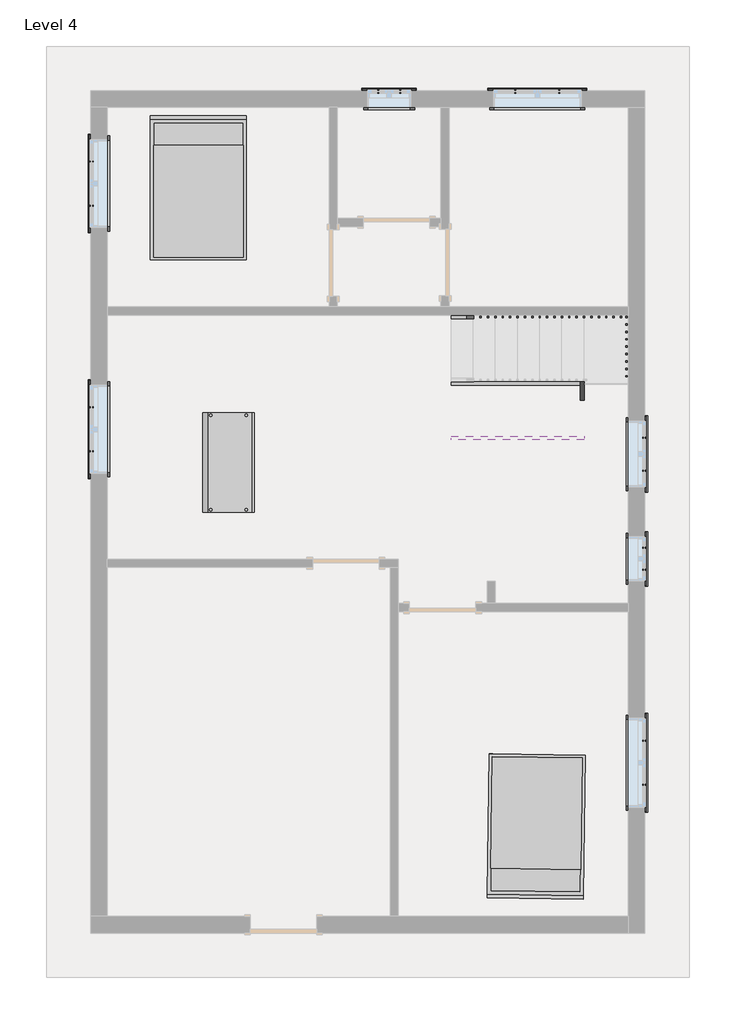
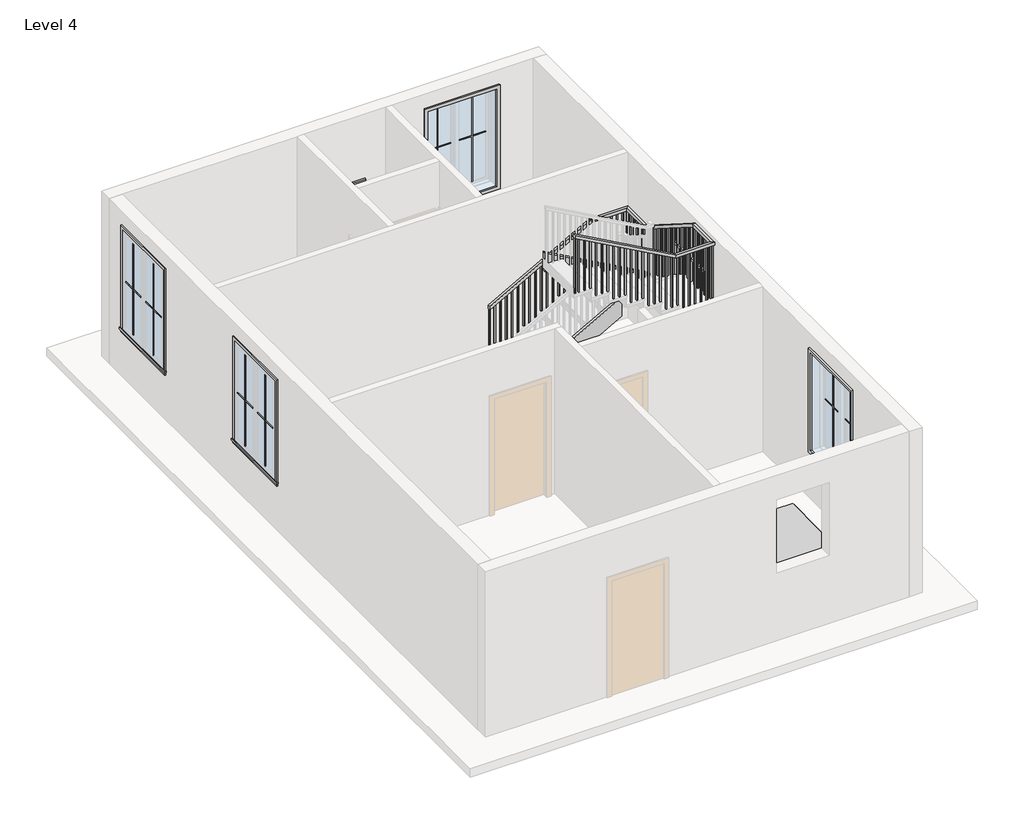
# One storey, part 2 of 2: 29 proxies, 3 members, 2 furniture elements, 1 railing.
"""IFC4 building model written with IfcOpenShell, lengths in millimetres."""

from ifc_helpers import new_model, si_unit, frame, origin, place, context, project, spatial, polyline, outline, extrude, faceted_brep, transform, mapped, element, save
from components import modern_coffee_table_17989_modern_coffee_table_17989_d3a860c8, muntin_pattern_2x2_muntin_pattern_2x2_2b4d9f72, muntin_pattern_2x2_muntin_pattern_2x2_ef995ed3, muntin_pattern_2x2_muntin_pattern_2x2_53152e2c, muntin_pattern_2x2_muntin_pattern_2x2_e8f3e573, muntin_pattern_2x2_muntin_pattern_2x2_9b64c8d5, muntin_pattern_2x2_muntin_pattern_2x2_d319fd2e, trim_window_exterior_flat_with_sill_b7e4d11c, trim_window_exterior_flat_with_sill_a665a915, trim_window_exterior_flat_with_sill_66148908, trim_window_interior_flat_picture_frame_936b8d2a, trim_window_interior_flat_picture_frame_d485c387, trim_window_interior_flat_picture_frame_d5b7f3a4, bed_17739_bed_17739_15c61121

model = new_model("IFC4")

# Units and contexts
model_context = context("Model", 3, world=origin())
ifc_project = project(units=[si_unit("LENGTHUNIT", "METRE", prefix="MILLI")], contexts=[model_context])

# Site, building, storey
site = spatial("IfcSite", under=ifc_project)
building = spatial("IfcBuilding", under=site)
storey = spatial("IfcBuildingStorey", under=building, Name="Level 4", Elevation=9144.0)

# Proxies
placement = place(None, origin())
modern_coffee_table_17989_modern_coffee_table_17989_shape = modern_coffee_table_17989_modern_coffee_table_17989_d3a860c8(model_context)
element("IfcBuildingElementProxy", 1, Name="Modern_Coffee_Table_17989 : Modern_Coffee_Table_17989", ObjectType="Modern_Coffee_Table_17989 : Modern_Coffee_Table_17989", at=placement, inside=storey, context=model_context, shape_type="MappedRepresentation", body=[
    mapped(modern_coffee_table_17989_modern_coffee_table_17989_shape, transform((3060.7, 9172.1823212, 9144.0), x_axis=(0.0, 1.0, 0.0), y_axis=(-1.0, 0.0, 0.0), z_axis=(0.0, 0.0, 1.0))),
])
muntin_pattern_2x2_muntin_pattern_2x2_shape = muntin_pattern_2x2_muntin_pattern_2x2_2b4d9f72(model_context)
element("IfcBuildingElementProxy", 2, Name="Muntin Pattern_2x2 : Muntin Pattern_2x2", ObjectType="Muntin Pattern_2x2 : Muntin Pattern_2x2", at=placement, inside=storey, context=model_context, shape_type="MappedRepresentation", body=[
    mapped(muntin_pattern_2x2_muntin_pattern_2x2_shape, transform((1533.525, 12477.4069306, 10128.25), x_axis=(0.0, 1.0, 0.0), y_axis=(-1.0, 0.0, 0.0), z_axis=(0.0, 0.0, 1.0))),
])
element("IfcBuildingElementProxy", 3, Name="Muntin Pattern_2x2 : Muntin Pattern_2x2", ObjectType="Muntin Pattern_2x2 : Muntin Pattern_2x2", at=placement, inside=storey, context=model_context, shape_type="MappedRepresentation", body=[
    mapped(muntin_pattern_2x2_muntin_pattern_2x2_shape, transform((7361.2375, 14045.8073212, 10128.25), x_axis=(1.0, 0.0, 0.0), y_axis=(0.0, 1.0, 0.0), z_axis=(0.0, 0.0, 1.0))),
])
element("IfcBuildingElementProxy", 4, Name="Muntin Pattern_2x2 : Muntin Pattern_2x2", ObjectType="Muntin Pattern_2x2 : Muntin Pattern_2x2", at=placement, inside=storey, context=model_context, shape_type="MappedRepresentation", body=[
    mapped(muntin_pattern_2x2_muntin_pattern_2x2_shape, transform((9134.475, 5119.2948212, 10128.25), x_axis=(0.0, -1.0, 0.0), y_axis=(1.0, 0.0, 0.0), z_axis=(0.0, 0.0, 1.0))),
])
element("IfcBuildingElementProxy", 5, Name="Muntin Pattern_2x2 : Muntin Pattern_2x2", ObjectType="Muntin Pattern_2x2 : Muntin Pattern_2x2", at=placement, inside=storey, context=model_context, shape_type="MappedRepresentation", body=[
    mapped(muntin_pattern_2x2_muntin_pattern_2x2_shape, transform((1533.525, 9097.5698212, 10128.25), x_axis=(0.0, 1.0, 0.0), y_axis=(-1.0, 0.0, 0.0), z_axis=(0.0, 0.0, 1.0))),
])
muntin_pattern_2x2_muntin_pattern_2x2_2_shape = muntin_pattern_2x2_muntin_pattern_2x2_ef995ed3(model_context)
element("IfcBuildingElementProxy", 6, Name="Muntin Pattern_2x2 : Muntin Pattern_2x2", ObjectType="Muntin Pattern_2x2 : Muntin Pattern_2x2", at=placement, inside=storey, context=model_context, shape_type="MappedRepresentation", body=[
    mapped(muntin_pattern_2x2_muntin_pattern_2x2_2_shape, transform((1533.525, 13083.8319306, 10128.25), x_axis=(0.0, -1.0, 0.0), y_axis=(1.0, 0.0, 0.0), z_axis=(0.0, 0.0, 1.0))),
])
element("IfcBuildingElementProxy", 7, Name="Muntin Pattern_2x2 : Muntin Pattern_2x2", ObjectType="Muntin Pattern_2x2 : Muntin Pattern_2x2", at=placement, inside=storey, context=model_context, shape_type="MappedRepresentation", body=[
    mapped(muntin_pattern_2x2_muntin_pattern_2x2_2_shape, transform((7967.6625, 14045.8073212, 10128.25), x_axis=(-1.0, 0.0, 0.0), y_axis=(0.0, -1.0, 0.0), z_axis=(0.0, 0.0, 1.0))),
])
element("IfcBuildingElementProxy", 8, Name="Muntin Pattern_2x2 : Muntin Pattern_2x2", ObjectType="Muntin Pattern_2x2 : Muntin Pattern_2x2", at=placement, inside=storey, context=model_context, shape_type="MappedRepresentation", body=[
    mapped(muntin_pattern_2x2_muntin_pattern_2x2_2_shape, transform((9134.475, 4512.8698212, 10128.25), x_axis=(0.0, 1.0, 0.0), y_axis=(-1.0, 0.0, 0.0), z_axis=(0.0, 0.0, 1.0))),
])
element("IfcBuildingElementProxy", 9, Name="Muntin Pattern_2x2 : Muntin Pattern_2x2", ObjectType="Muntin Pattern_2x2 : Muntin Pattern_2x2", at=placement, inside=storey, context=model_context, shape_type="MappedRepresentation", body=[
    mapped(muntin_pattern_2x2_muntin_pattern_2x2_2_shape, transform((1533.525, 9703.9948212, 10128.25), x_axis=(0.0, -1.0, 0.0), y_axis=(1.0, 0.0, 0.0), z_axis=(0.0, 0.0, 1.0))),
])
muntin_pattern_2x2_muntin_pattern_2x2_3_shape = muntin_pattern_2x2_muntin_pattern_2x2_53152e2c(model_context)
element("IfcBuildingElementProxy", 10, Name="Muntin Pattern_2x2 : Muntin Pattern_2x2", ObjectType="Muntin Pattern_2x2 : Muntin Pattern_2x2", at=placement, inside=storey, context=model_context, shape_type="MappedRepresentation", body=[
    mapped(muntin_pattern_2x2_muntin_pattern_2x2_3_shape, transform((9134.475, 7771.2135712, 10128.25), x_axis=(0.0, -1.0, 0.0), y_axis=(1.0, 0.0, 0.0), z_axis=(0.0, 0.0, 1.0))),
])
element("IfcBuildingElementProxy", 11, Name="Muntin Pattern_2x2 : Muntin Pattern_2x2", ObjectType="Muntin Pattern_2x2 : Muntin Pattern_2x2", at=placement, inside=storey, context=model_context, shape_type="MappedRepresentation", body=[
    mapped(muntin_pattern_2x2_muntin_pattern_2x2_3_shape, transform((5475.2875, 14045.8073212, 10128.25), x_axis=(1.0, 0.0, 0.0), y_axis=(0.0, 1.0, 0.0), z_axis=(0.0, 0.0, 1.0))),
])
muntin_pattern_2x2_muntin_pattern_2x2_4_shape = muntin_pattern_2x2_muntin_pattern_2x2_e8f3e573(model_context)
element("IfcBuildingElementProxy", 12, Name="Muntin Pattern_2x2 : Muntin Pattern_2x2", ObjectType="Muntin Pattern_2x2 : Muntin Pattern_2x2", at=placement, inside=storey, context=model_context, shape_type="MappedRepresentation", body=[
    mapped(muntin_pattern_2x2_muntin_pattern_2x2_4_shape, transform((9134.475, 7469.5885712, 10128.25), x_axis=(0.0, 1.0, 0.0), y_axis=(-1.0, 0.0, 0.0), z_axis=(0.0, 0.0, 1.0))),
])
element("IfcBuildingElementProxy", 13, Name="Muntin Pattern_2x2 : Muntin Pattern_2x2", ObjectType="Muntin Pattern_2x2 : Muntin Pattern_2x2", at=placement, inside=storey, context=model_context, shape_type="MappedRepresentation", body=[
    mapped(muntin_pattern_2x2_muntin_pattern_2x2_4_shape, transform((5776.9125, 14045.8073212, 10128.25), x_axis=(-1.0, 0.0, 0.0), y_axis=(0.0, -1.0, 0.0), z_axis=(0.0, 0.0, 1.0))),
])
muntin_pattern_2x2_muntin_pattern_2x2_5_shape = muntin_pattern_2x2_muntin_pattern_2x2_9b64c8d5(model_context)
element("IfcBuildingElementProxy", 14, Name="Muntin Pattern_2x2 : Muntin Pattern_2x2", ObjectType="Muntin Pattern_2x2 : Muntin Pattern_2x2", at=placement, inside=storey, context=model_context, shape_type="MappedRepresentation", body=[
    mapped(muntin_pattern_2x2_muntin_pattern_2x2_5_shape, transform((9134.475, 9287.1024384, 10128.25), x_axis=(0.0, -1.0, 0.0), y_axis=(1.0, 0.0, 0.0), z_axis=(0.0, 0.0, 1.0))),
])
muntin_pattern_2x2_muntin_pattern_2x2_6_shape = muntin_pattern_2x2_muntin_pattern_2x2_d319fd2e(model_context)
element("IfcBuildingElementProxy", 15, Name="Muntin Pattern_2x2 : Muntin Pattern_2x2", ObjectType="Muntin Pattern_2x2 : Muntin Pattern_2x2", at=placement, inside=storey, context=model_context, shape_type="MappedRepresentation", body=[
    mapped(muntin_pattern_2x2_muntin_pattern_2x2_6_shape, transform((9134.475, 8833.0774384, 10128.25), x_axis=(0.0, 1.0, 0.0), y_axis=(-1.0, 0.0, 0.0), z_axis=(0.0, 0.0, 1.0))),
])
trim_window_exterior_flat_with_sill_shape = trim_window_exterior_flat_with_sill_b7e4d11c(model_context)
element("IfcBuildingElementProxy", 16, Name="Trim-Window-Exterior-Flat : with Sill", ObjectType="Trim-Window-Exterior-Flat : with Sill", at=placement, inside=storey, context=model_context, shape_type="MappedRepresentation", body=[
    mapped(trim_window_exterior_flat_with_sill_shape, transform((1524.0, 12780.6194306, 11887.2), x_axis=(0.0, -1.0, 0.0), y_axis=(0.0, 0.0, 1.0), z_axis=(-1.0, 0.0, 0.0))),
])
element("IfcBuildingElementProxy", 17, Name="Trim-Window-Exterior-Flat : with Sill", ObjectType="Trim-Window-Exterior-Flat : with Sill", at=placement, inside=storey, context=model_context, shape_type="MappedRepresentation", body=[
    mapped(trim_window_exterior_flat_with_sill_shape, transform((7664.45, 14055.3323212, 11887.2), x_axis=(-1.0, 0.0, 0.0), y_axis=(0.0, 0.0, 1.0), z_axis=(0.0, 1.0, 0.0))),
])
element("IfcBuildingElementProxy", 18, Name="Trim-Window-Exterior-Flat : with Sill", ObjectType="Trim-Window-Exterior-Flat : with Sill", at=placement, inside=storey, context=model_context, shape_type="MappedRepresentation", body=[
    mapped(trim_window_exterior_flat_with_sill_shape, transform((9144.0, 4816.0823212, 11887.2), x_axis=(0.0, 1.0, 0.0), y_axis=(0.0, 0.0, 1.0), z_axis=(1.0, 0.0, 0.0))),
])
element("IfcBuildingElementProxy", 19, Name="Trim-Window-Exterior-Flat : with Sill", ObjectType="Trim-Window-Exterior-Flat : with Sill", at=placement, inside=storey, context=model_context, shape_type="MappedRepresentation", body=[
    mapped(trim_window_exterior_flat_with_sill_shape, transform((1524.0, 9400.7823212, 11887.2), x_axis=(0.0, -1.0, 0.0), y_axis=(0.0, 0.0, 1.0), z_axis=(-1.0, 0.0, 0.0))),
])
trim_window_exterior_flat_with_sill_2_shape = trim_window_exterior_flat_with_sill_a665a915(model_context)
element("IfcBuildingElementProxy", 20, Name="Trim-Window-Exterior-Flat : with Sill", ObjectType="Trim-Window-Exterior-Flat : with Sill", at=placement, inside=storey, context=model_context, shape_type="MappedRepresentation", body=[
    mapped(trim_window_exterior_flat_with_sill_2_shape, transform((9144.0, 7620.4010712, 10972.8), x_axis=(0.0, 1.0, 0.0), y_axis=(0.0, 0.0, 1.0), z_axis=(1.0, 0.0, 0.0))),
])
element("IfcBuildingElementProxy", 21, Name="Trim-Window-Exterior-Flat : with Sill", ObjectType="Trim-Window-Exterior-Flat : with Sill", at=placement, inside=storey, context=model_context, shape_type="MappedRepresentation", body=[
    mapped(trim_window_exterior_flat_with_sill_2_shape, transform((5626.1, 14055.3323212, 10972.8), x_axis=(-1.0, 0.0, 0.0), y_axis=(0.0, 0.0, 1.0), z_axis=(0.0, 1.0, 0.0))),
])
trim_window_exterior_flat_with_sill_3_shape = trim_window_exterior_flat_with_sill_66148908(model_context)
element("IfcBuildingElementProxy", 22, Name="Trim-Window-Exterior-Flat : with Sill", ObjectType="Trim-Window-Exterior-Flat : with Sill", at=placement, inside=storey, context=model_context, shape_type="MappedRepresentation", body=[
    mapped(trim_window_exterior_flat_with_sill_3_shape, transform((9144.0, 9060.0899384, 11404.6), x_axis=(0.0, 1.0, 0.0), y_axis=(0.0, 0.0, 1.0), z_axis=(1.0, 0.0, 0.0))),
])
trim_window_interior_flat_picture_frame_shape = trim_window_interior_flat_picture_frame_936b8d2a(model_context)
element("IfcBuildingElementProxy", 23, Name="Trim-Window-Interior-Flat : Picture Frame", ObjectType="Trim-Window-Interior-Flat : Picture Frame", at=placement, inside=storey, context=model_context, shape_type="MappedRepresentation", body=[
    mapped(trim_window_interior_flat_picture_frame_shape, transform((1752.6, 12780.6194306, 11887.2), x_axis=(0.0, 1.0, 0.0), y_axis=(0.0, 0.0, 1.0), z_axis=(1.0, 0.0, 0.0))),
])
element("IfcBuildingElementProxy", 24, Name="Trim-Window-Interior-Flat : Picture Frame", ObjectType="Trim-Window-Interior-Flat : Picture Frame", at=placement, inside=storey, context=model_context, shape_type="MappedRepresentation", body=[
    mapped(trim_window_interior_flat_picture_frame_shape, transform((7664.45, 13826.7323212, 11887.2), x_axis=(1.0, 0.0, 0.0), y_axis=(0.0, 0.0, 1.0), z_axis=(0.0, -1.0, 0.0))),
])
element("IfcBuildingElementProxy", 25, Name="Trim-Window-Interior-Flat : Picture Frame", ObjectType="Trim-Window-Interior-Flat : Picture Frame", at=placement, inside=storey, context=model_context, shape_type="MappedRepresentation", body=[
    mapped(trim_window_interior_flat_picture_frame_shape, transform((8915.4, 4816.0823212, 11887.2), x_axis=(0.0, -1.0, 0.0), y_axis=(0.0, 0.0, 1.0), z_axis=(-1.0, 0.0, 0.0))),
])
element("IfcBuildingElementProxy", 26, Name="Trim-Window-Interior-Flat : Picture Frame", ObjectType="Trim-Window-Interior-Flat : Picture Frame", at=placement, inside=storey, context=model_context, shape_type="MappedRepresentation", body=[
    mapped(trim_window_interior_flat_picture_frame_shape, transform((1752.6, 9400.7823212, 11887.2), x_axis=(0.0, 1.0, 0.0), y_axis=(0.0, 0.0, 1.0), z_axis=(1.0, 0.0, 0.0))),
])
trim_window_interior_flat_picture_frame_2_shape = trim_window_interior_flat_picture_frame_d485c387(model_context)
element("IfcBuildingElementProxy", 27, Name="Trim-Window-Interior-Flat : Picture Frame", ObjectType="Trim-Window-Interior-Flat : Picture Frame", at=placement, inside=storey, context=model_context, shape_type="MappedRepresentation", body=[
    mapped(trim_window_interior_flat_picture_frame_2_shape, transform((8915.4, 7620.4010712, 10972.8), x_axis=(0.0, -1.0, 0.0), y_axis=(0.0, 0.0, 1.0), z_axis=(-1.0, 0.0, 0.0))),
])
element("IfcBuildingElementProxy", 28, Name="Trim-Window-Interior-Flat : Picture Frame", ObjectType="Trim-Window-Interior-Flat : Picture Frame", at=placement, inside=storey, context=model_context, shape_type="MappedRepresentation", body=[
    mapped(trim_window_interior_flat_picture_frame_2_shape, transform((5626.1, 13826.7323212, 10972.8), x_axis=(1.0, 0.0, 0.0), y_axis=(0.0, 0.0, 1.0), z_axis=(0.0, -1.0, 0.0))),
])
trim_window_interior_flat_picture_frame_3_shape = trim_window_interior_flat_picture_frame_d5b7f3a4(model_context)
element("IfcBuildingElementProxy", 29, Name="Trim-Window-Interior-Flat : Picture Frame", ObjectType="Trim-Window-Interior-Flat : Picture Frame", at=placement, inside=storey, context=model_context, shape_type="MappedRepresentation", body=[
    mapped(trim_window_interior_flat_picture_frame_3_shape, transform((8915.4, 9060.0899384, 11404.6), x_axis=(0.0, -1.0, 0.0), y_axis=(0.0, 0.0, 1.0), z_axis=(-1.0, 0.0, 0.0))),
])

# Furniture
bed_17739_bed_17739_shape = bed_17739_bed_17739_15c61121(model_context)
element("IfcFurniture", 30, ObjectType="Bed_17739 : Bed_17739", at=placement, inside=storey, context=model_context, shape_type="MappedRepresentation", body=[
    mapped(bed_17739_bed_17739_shape, transform((3003.55, 12696.4323212, 9144.0), x_axis=(1.0, 0.0, 0.0), y_axis=(0.0, 1.0, 0.0), z_axis=(0.0, 0.0, 1.0))),
])
element("IfcFurniture", 31, ObjectType="Bed_17739 : Bed_17739", at=placement, inside=storey, context=model_context, shape_type="MappedRepresentation", body=[
    mapped(bed_17739_bed_17739_shape, transform((7650.1504891, 3963.5673274, 9144.0), x_axis=(-0.9999063358908578, 0.013686469424921632, 0.0), y_axis=(-0.013686469424921632, -0.9999063358908578, 0.0), z_axis=(0.0, 0.0, 1.0))),
])

# Members
element("IfcMember", 32, ObjectType="Stringer - 2\" Width", at=placement, inside=storey, context=model_context, shape_type="SweptSolid", body=[
    extrude(outline(polyline([(9351.5983948, 6477.0), (9144.0, 6477.0), (9144.0, 6730.9445028), (9990.6974984, 8255.0), (10339.3761726, 8255.0), (9351.5983948, 6477.0)])), frame((0.0, 10004.0323212, 0.0), z_axis=(0.0, 1.0, 0.0), x_axis=(0.0, 0.0, 1.0)), (0.0, 0.0, 1.0), 50.8),
])
element("IfcMember", 33, ObjectType="Stringer - 2\" Width", at=placement, inside=storey, context=model_context, shape_type="SweptSolid", body=[
    extrude(outline(polyline([(10054.8323212, 10544.2030053), (10054.8323212, 10183.1566026), (9305.5323212, 10658.9026344), (9305.5323212, 11019.949037), (10054.8323212, 10544.2030053)])), frame((8255.0, 0.0, 0.0), z_axis=(1.0, 0.0, 0.0), x_axis=(0.0, 1.0, 0.0)), (0.0, 0.0, 1.0), 50.8),
])
element("IfcMember", 34, ObjectType="Stringer - 2\" Width", at=placement, inside=storey, context=model_context, shape_type="SweptSolid", body=[
    extrude(outline(polyline([(10865.5863873, 8305.8), (11214.2650614, 8305.8), (12230.2650614, 6477.0), (11881.5863873, 6477.0), (10865.5863873, 8305.8)])), frame((0.0, 9254.7323212, 0.0), z_axis=(0.0, 1.0, 0.0), x_axis=(0.0, 0.0, 1.0)), (0.0, 0.0, 1.0), 50.8),
])

# Railing
element("IfcRailing", 35, ObjectType="Handrail - Rectangular", at=placement, inside=storey, context=model_context, shape_type="SolidModel", body=[
    faceted_brep([(6477.0, 10969.2323212, 10227.7333333), (6477.0, 10969.2323212, 10169.620221), (6477.0, 10918.4323212, 10169.620221), (6477.0, 10918.4323212, 10227.7333333), (8242.3, 10969.2323212, 11208.4555556), (8255.4636022, 10969.2323212, 11157.6555556), (8255.4636022, 10918.4323212, 11157.6555556), (8242.3, 10918.4323212, 11208.4555556), (8915.4, 10969.2323212, 11208.4555556), (8915.4, 10969.2323212, 11157.6555556), (8864.6, 10918.4323212, 11157.6555556), (8864.6, 10918.4323212, 11208.4555556), (8915.4, 10377.0948212, 11208.4555556), (8915.4, 10362.3301405, 11157.6555556), (8864.6, 10362.3301405, 11157.6555556), (8864.6, 10377.0948212, 11208.4555556), (8915.4, 8932.4698212, 12125.6777778), (8915.4, 8917.7051405, 12074.8777778), (8864.6, 8917.7051405, 12074.8777778), (8864.6, 8932.4698212, 12125.6777778), (8915.4, 8340.3323212, 12125.6777778), (8915.4, 8340.3323212, 12074.8777778), (8864.6, 8391.1323212, 12074.8777778), (8864.6, 8391.1323212, 12125.6777778), (8242.3, 8340.3323212, 12125.6777778), (8229.1363978, 8340.3323212, 12074.8777778), (8229.1363978, 8391.1323212, 12074.8777778), (8242.3, 8391.1323212, 12125.6777778), (6477.0, 8340.3323212, 13106.4), (6477.0, 8391.1323212, 13106.4), (6477.0, 8391.1323212, 13048.2868876), (6477.0, 8340.3323212, 13048.2868876)], [[[0, 1, 2, 3]], [[1, 0, 4, 5]], [[2, 1, 5, 6]], [[3, 2, 6, 7]], [[0, 3, 7, 4]], [[5, 4, 8, 9]], [[6, 5, 9, 10]], [[7, 6, 10, 11]], [[4, 7, 11, 8]], [[9, 8, 12, 13]], [[10, 9, 13, 14]], [[11, 10, 14, 15]], [[8, 11, 15, 12]], [[13, 12, 16, 17]], [[14, 13, 17, 18]], [[15, 14, 18, 19]], [[12, 15, 19, 16]], [[17, 16, 20, 21]], [[18, 17, 21, 22]], [[19, 18, 22, 23]], [[16, 19, 23, 20]], [[21, 20, 24, 25]], [[22, 21, 25, 26]], [[23, 22, 26, 27]], [[20, 23, 27, 24]], [[28, 29, 30, 31]], [[25, 24, 28, 31]], [[26, 25, 31, 30]], [[27, 26, 30, 29]], [[24, 27, 29, 28]]]),
    extrude(outline(polyline([(13011.245221, 6543.675), (12022.6666667, 6543.675), (12022.6666667, 6562.725), (13000.6618876, 6562.725), (13011.245221, 6543.675)])), frame((0.0, 8356.2073212, 0.0), z_axis=(0.0, 1.0, 0.0), x_axis=(0.0, 0.0, 1.0)), (0.0, 0.0, 1.0), 19.05),
    extrude(outline(polyline([(12954.8007765, 6645.275), (12022.6666667, 6645.275), (12022.6666667, 6664.325), (12944.2174432, 6664.325), (12954.8007765, 6645.275)])), frame((0.0, 8356.2073212, 0.0), z_axis=(0.0, 1.0, 0.0), x_axis=(0.0, 0.0, 1.0)), (0.0, 0.0, 1.0), 19.05),
    extrude(outline(polyline([(12898.3563321, 6746.875), (12022.6666667, 6746.875), (12022.6666667, 6765.925), (12887.7729988, 6765.925), (12898.3563321, 6746.875)])), frame((0.0, 8356.2073212, 0.0), z_axis=(0.0, 1.0, 0.0), x_axis=(0.0, 0.0, 1.0)), (0.0, 0.0, 1.0), 19.05),
    extrude(outline(polyline([(12841.9118876, 6848.475), (11853.3333333, 6848.475), (11853.3333333, 6867.525), (12831.3285543, 6867.525), (12841.9118876, 6848.475)])), frame((0.0, 8356.2073212, 0.0), z_axis=(0.0, 1.0, 0.0), x_axis=(0.0, 0.0, 1.0)), (0.0, 0.0, 1.0), 19.05),
    extrude(outline(polyline([(12785.4674432, 6950.075), (11853.3333333, 6950.075), (11853.3333333, 6969.125), (12774.8841099, 6969.125), (12785.4674432, 6950.075)])), frame((0.0, 8356.2073212, 0.0), z_axis=(0.0, 1.0, 0.0), x_axis=(0.0, 0.0, 1.0)), (0.0, 0.0, 1.0), 19.05),
    extrude(outline(polyline([(12729.0229988, 7051.675), (11853.3333333, 7051.675), (11853.3333333, 7070.725), (12718.4396654, 7070.725), (12729.0229988, 7051.675)])), frame((0.0, 8356.2073212, 0.0), z_axis=(0.0, 1.0, 0.0), x_axis=(0.0, 0.0, 1.0)), (0.0, 0.0, 1.0), 19.05),
    extrude(outline(polyline([(12672.5785543, 7153.275), (11684.0, 7153.275), (11684.0, 7172.325), (12661.995221, 7172.325), (12672.5785543, 7153.275)])), frame((0.0, 8356.2073212, 0.0), z_axis=(0.0, 1.0, 0.0), x_axis=(0.0, 0.0, 1.0)), (0.0, 0.0, 1.0), 19.05),
    extrude(outline(polyline([(12616.1341099, 7254.875), (11684.0, 7254.875), (11684.0, 7273.925), (12605.5507765, 7273.925), (12616.1341099, 7254.875)])), frame((0.0, 8356.2073212, 0.0), z_axis=(0.0, 1.0, 0.0), x_axis=(0.0, 0.0, 1.0)), (0.0, 0.0, 1.0), 19.05),
    extrude(outline(polyline([(12559.6896654, 7356.475), (11684.0, 7356.475), (11684.0, 7375.525), (12549.1063321, 7375.525), (12559.6896654, 7356.475)])), frame((0.0, 8356.2073212, 0.0), z_axis=(0.0, 1.0, 0.0), x_axis=(0.0, 0.0, 1.0)), (0.0, 0.0, 1.0), 19.05),
    extrude(outline(polyline([(12503.245221, 7458.075), (11514.6666667, 7458.075), (11514.6666667, 7477.125), (12492.6618876, 7477.125), (12503.245221, 7458.075)])), frame((0.0, 8356.2073212, 0.0), z_axis=(0.0, 1.0, 0.0), x_axis=(0.0, 0.0, 1.0)), (0.0, 0.0, 1.0), 19.05),
    extrude(outline(polyline([(12446.8007765, 7559.675), (11514.6666667, 7559.675), (11514.6666667, 7578.725), (12436.2174432, 7578.725), (12446.8007765, 7559.675)])), frame((0.0, 8356.2073212, 0.0), z_axis=(0.0, 1.0, 0.0), x_axis=(0.0, 0.0, 1.0)), (0.0, 0.0, 1.0), 19.05),
    extrude(outline(polyline([(12390.3563321, 7661.275), (11514.6666667, 7661.275), (11514.6666667, 7680.325), (12379.7729988, 7680.325), (12390.3563321, 7661.275)])), frame((0.0, 8356.2073212, 0.0), z_axis=(0.0, 1.0, 0.0), x_axis=(0.0, 0.0, 1.0)), (0.0, 0.0, 1.0), 19.05),
    extrude(outline(polyline([(12333.9118876, 7762.875), (11345.3333333, 7762.875), (11345.3333333, 7781.925), (12323.3285543, 7781.925), (12333.9118876, 7762.875)])), frame((0.0, 8356.2073212, 0.0), z_axis=(0.0, 1.0, 0.0), x_axis=(0.0, 0.0, 1.0)), (0.0, 0.0, 1.0), 19.05),
    extrude(outline(polyline([(12277.4674432, 7864.475), (11345.3333333, 7864.475), (11345.3333333, 7883.525), (12266.8841099, 7883.525), (12277.4674432, 7864.475)])), frame((0.0, 8356.2073212, 0.0), z_axis=(0.0, 1.0, 0.0), x_axis=(0.0, 0.0, 1.0)), (0.0, 0.0, 1.0), 19.05),
    extrude(outline(polyline([(12221.0229988, 7966.075), (11345.3333333, 7966.075), (11345.3333333, 7985.125), (12210.4396654, 7985.125), (12221.0229988, 7966.075)])), frame((0.0, 8356.2073212, 0.0), z_axis=(0.0, 1.0, 0.0), x_axis=(0.0, 0.0, 1.0)), (0.0, 0.0, 1.0), 19.05),
    extrude(outline(polyline([(12164.5785543, 8067.675), (11176.0, 8067.675), (11176.0, 8086.725), (12153.995221, 8086.725), (12164.5785543, 8067.675)])), frame((0.0, 8356.2073212, 0.0), z_axis=(0.0, 1.0, 0.0), x_axis=(0.0, 0.0, 1.0)), (0.0, 0.0, 1.0), 19.05),
    extrude(outline(polyline([(12108.1341099, 8169.275), (11176.0, 8169.275), (11176.0, 8188.325), (12097.5507765, 8188.325), (12108.1341099, 8169.275)])), frame((0.0, 8356.2073212, 0.0), z_axis=(0.0, 1.0, 0.0), x_axis=(0.0, 0.0, 1.0)), (0.0, 0.0, 1.0), 19.05),
    extrude(outline(polyline([(8289.925, 8356.2073212), (8270.875, 8356.2073212), (8270.875, 8375.2573212), (8289.925, 8375.2573212), (8289.925, 8356.2073212)])), frame((0.0, 0.0, 11176.0), z_axis=(0.0, 0.0, 1.0), x_axis=(1.0, 0.0, 0.0)), (0.0, 0.0, 1.0), 898.8777778),
    extrude(outline(polyline([(8391.525, 8356.2073212), (8372.475, 8356.2073212), (8372.475, 8375.2573212), (8391.525, 8375.2573212), (8391.525, 8356.2073212)])), frame((0.0, 0.0, 11006.6666667), z_axis=(0.0, 0.0, 1.0), x_axis=(1.0, 0.0, 0.0)), (0.0, 0.0, 1.0), 1068.2111111),
    extrude(outline(polyline([(8493.125, 8356.2073212), (8474.075, 8356.2073212), (8474.075, 8375.2573212), (8493.125, 8375.2573212), (8493.125, 8356.2073212)])), frame((0.0, 0.0, 11006.6666667), z_axis=(0.0, 0.0, 1.0), x_axis=(1.0, 0.0, 0.0)), (0.0, 0.0, 1.0), 1068.2111111),
    extrude(outline(polyline([(8594.725, 8356.2073212), (8575.675, 8356.2073212), (8575.675, 8375.2573212), (8594.725, 8375.2573212), (8594.725, 8356.2073212)])), frame((0.0, 0.0, 11006.6666667), z_axis=(0.0, 0.0, 1.0), x_axis=(1.0, 0.0, 0.0)), (0.0, 0.0, 1.0), 1068.2111111),
    extrude(outline(polyline([(8696.325, 8356.2073212), (8677.275, 8356.2073212), (8677.275, 8375.2573212), (8696.325, 8375.2573212), (8696.325, 8356.2073212)])), frame((0.0, 0.0, 11006.6666667), z_axis=(0.0, 0.0, 1.0), x_axis=(1.0, 0.0, 0.0)), (0.0, 0.0, 1.0), 1068.2111111),
    extrude(outline(polyline([(8797.925, 8356.2073212), (8778.875, 8356.2073212), (8778.875, 8375.2573212), (8797.925, 8375.2573212), (8797.925, 8356.2073212)])), frame((0.0, 0.0, 11006.6666667), z_axis=(0.0, 0.0, 1.0), x_axis=(1.0, 0.0, 0.0)), (0.0, 0.0, 1.0), 1068.2111111),
    extrude(outline(polyline([(8899.525, 8413.3573212), (8899.525, 8394.3073212), (8880.475, 8394.3073212), (8880.475, 8413.3573212), (8899.525, 8413.3573212)])), frame((0.0, 0.0, 11006.6666667), z_axis=(0.0, 0.0, 1.0), x_axis=(1.0, 0.0, 0.0)), (0.0, 0.0, 1.0), 1068.2111111),
    extrude(outline(polyline([(8899.525, 8514.9573212), (8899.525, 8495.9073212), (8880.475, 8495.9073212), (8880.475, 8514.9573212), (8899.525, 8514.9573212)])), frame((0.0, 0.0, 11006.6666667), z_axis=(0.0, 0.0, 1.0), x_axis=(1.0, 0.0, 0.0)), (0.0, 0.0, 1.0), 1068.2111111),
    extrude(outline(polyline([(8899.525, 8616.5573212), (8899.525, 8597.5073212), (8880.475, 8597.5073212), (8880.475, 8616.5573212), (8899.525, 8616.5573212)])), frame((0.0, 0.0, 11006.6666667), z_axis=(0.0, 0.0, 1.0), x_axis=(1.0, 0.0, 0.0)), (0.0, 0.0, 1.0), 1068.2111111),
    extrude(outline(polyline([(8899.525, 8718.1573212), (8899.525, 8699.1073212), (8880.475, 8699.1073212), (8880.475, 8718.1573212), (8899.525, 8718.1573212)])), frame((0.0, 0.0, 11006.6666667), z_axis=(0.0, 0.0, 1.0), x_axis=(1.0, 0.0, 0.0)), (0.0, 0.0, 1.0), 1068.2111111),
    extrude(outline(polyline([(8899.525, 8819.7573212), (8899.525, 8800.7073212), (8880.475, 8800.7073212), (8880.475, 8819.7573212), (8899.525, 8819.7573212)])), frame((0.0, 0.0, 11006.6666667), z_axis=(0.0, 0.0, 1.0), x_axis=(1.0, 0.0, 0.0)), (0.0, 0.0, 1.0), 1068.2111111),
    extrude(outline(polyline([(8899.525, 8921.3573212), (8899.525, 8902.3073212), (8880.475, 8902.3073212), (8880.475, 8921.3573212), (8899.525, 8921.3573212)])), frame((0.0, 0.0, 11006.6666667), z_axis=(0.0, 0.0, 1.0), x_axis=(1.0, 0.0, 0.0)), (0.0, 0.0, 1.0), 1068.2111111),
    extrude(outline(polyline([(9022.9573212, 12008.0509964), (9022.9573212, 11006.6666667), (9003.9073212, 11006.6666667), (9003.9073212, 12020.1462345), (9022.9573212, 12008.0509964)])), frame((8880.475, 0.0, 0.0), z_axis=(1.0, 0.0, 0.0), x_axis=(0.0, 1.0, 0.0)), (0.0, 0.0, 1.0), 19.05),
    extrude(outline(polyline([(9124.5573212, 11943.5430599), (9124.5573212, 11006.6666667), (9105.5073212, 11006.6666667), (9105.5073212, 11955.638298), (9124.5573212, 11943.5430599)])), frame((8880.475, 0.0, 0.0), z_axis=(1.0, 0.0, 0.0), x_axis=(0.0, 1.0, 0.0)), (0.0, 0.0, 1.0), 19.05),
    extrude(outline(polyline([(9226.1573212, 11879.0351234), (9226.1573212, 11006.6666667), (9207.1073212, 11006.6666667), (9207.1073212, 11891.1303615), (9226.1573212, 11879.0351234)])), frame((8880.475, 0.0, 0.0), z_axis=(1.0, 0.0, 0.0), x_axis=(0.0, 1.0, 0.0)), (0.0, 0.0, 1.0), 19.05),
    extrude(outline(polyline([(9327.7573212, 11814.5271869), (9327.7573212, 10837.3333333), (9308.7073212, 10837.3333333), (9308.7073212, 11826.622425), (9327.7573212, 11814.5271869)])), frame((8880.475, 0.0, 0.0), z_axis=(1.0, 0.0, 0.0), x_axis=(0.0, 1.0, 0.0)), (0.0, 0.0, 1.0), 19.05),
    extrude(outline(polyline([(9429.3573212, 11750.0192504), (9429.3573212, 10837.3333333), (9410.3073212, 10837.3333333), (9410.3073212, 11762.1144884), (9429.3573212, 11750.0192504)])), frame((8880.475, 0.0, 0.0), z_axis=(1.0, 0.0, 0.0), x_axis=(0.0, 1.0, 0.0)), (0.0, 0.0, 1.0), 19.05),
    extrude(outline(polyline([(9530.9573212, 11685.5113138), (9530.9573212, 10668.0), (9511.9073212, 10668.0), (9511.9073212, 11697.6065519), (9530.9573212, 11685.5113138)])), frame((8880.475, 0.0, 0.0), z_axis=(1.0, 0.0, 0.0), x_axis=(0.0, 1.0, 0.0)), (0.0, 0.0, 1.0), 19.05),
    extrude(outline(polyline([(9632.5573212, 11621.0033773), (9632.5573212, 10668.0), (9613.5073212, 10668.0), (9613.5073212, 11633.0986154), (9632.5573212, 11621.0033773)])), frame((8880.475, 0.0, 0.0), z_axis=(1.0, 0.0, 0.0), x_axis=(0.0, 1.0, 0.0)), (0.0, 0.0, 1.0), 19.05),
    extrude(outline(polyline([(9734.1573212, 11556.4954408), (9734.1573212, 10668.0), (9715.1073212, 10668.0), (9715.1073212, 11568.5906789), (9734.1573212, 11556.4954408)])), frame((8880.475, 0.0, 0.0), z_axis=(1.0, 0.0, 0.0), x_axis=(0.0, 1.0, 0.0)), (0.0, 0.0, 1.0), 19.05),
    extrude(outline(polyline([(9835.7573212, 11491.9875043), (9835.7573212, 10498.6666667), (9816.7073212, 10498.6666667), (9816.7073212, 11504.0827424), (9835.7573212, 11491.9875043)])), frame((8880.475, 0.0, 0.0), z_axis=(1.0, 0.0, 0.0), x_axis=(0.0, 1.0, 0.0)), (0.0, 0.0, 1.0), 19.05),
    extrude(outline(polyline([(9937.3573212, 11427.4795678), (9937.3573212, 10498.6666667), (9918.3073212, 10498.6666667), (9918.3073212, 11439.5748059), (9937.3573212, 11427.4795678)])), frame((8880.475, 0.0, 0.0), z_axis=(1.0, 0.0, 0.0), x_axis=(0.0, 1.0, 0.0)), (0.0, 0.0, 1.0), 19.05),
    extrude(outline(polyline([(10038.9573212, 11362.9716313), (10038.9573212, 10498.6666667), (10019.9073212, 10498.6666667), (10019.9073212, 11375.0668694), (10038.9573212, 11362.9716313)])), frame((8880.475, 0.0, 0.0), z_axis=(1.0, 0.0, 0.0), x_axis=(0.0, 1.0, 0.0)), (0.0, 0.0, 1.0), 19.05),
    extrude(outline(polyline([(10140.5573212, 11298.4636948), (10140.5573212, 10329.3333333), (10121.5073212, 10329.3333333), (10121.5073212, 11310.5589329), (10140.5573212, 11298.4636948)])), frame((8880.475, 0.0, 0.0), z_axis=(1.0, 0.0, 0.0), x_axis=(0.0, 1.0, 0.0)), (0.0, 0.0, 1.0), 19.05),
    extrude(outline(polyline([(10242.1573212, 11233.9557583), (10242.1573212, 10329.3333333), (10223.1073212, 10329.3333333), (10223.1073212, 11246.0509964), (10242.1573212, 11233.9557583)])), frame((8880.475, 0.0, 0.0), z_axis=(1.0, 0.0, 0.0), x_axis=(0.0, 1.0, 0.0)), (0.0, 0.0, 1.0), 19.05),
    extrude(outline(polyline([(10343.7573212, 11169.4478218), (10343.7573212, 10329.3333333), (10324.7073212, 10329.3333333), (10324.7073212, 11181.5430599), (10343.7573212, 11169.4478218)])), frame((8880.475, 0.0, 0.0), z_axis=(1.0, 0.0, 0.0), x_axis=(0.0, 1.0, 0.0)), (0.0, 0.0, 1.0), 19.05),
    extrude(outline(polyline([(8899.525, 10445.3573212), (8899.525, 10426.3073212), (8880.475, 10426.3073212), (8880.475, 10445.3573212), (8899.525, 10445.3573212)])), frame((0.0, 0.0, 10329.3333333), z_axis=(0.0, 0.0, 1.0), x_axis=(1.0, 0.0, 0.0)), (0.0, 0.0, 1.0), 828.3222222),
    extrude(outline(polyline([(8899.525, 10546.9573212), (8899.525, 10527.9073212), (8880.475, 10527.9073212), (8880.475, 10546.9573212), (8899.525, 10546.9573212)])), frame((0.0, 0.0, 10329.3333333), z_axis=(0.0, 0.0, 1.0), x_axis=(1.0, 0.0, 0.0)), (0.0, 0.0, 1.0), 828.3222222),
    extrude(outline(polyline([(8899.525, 10648.5573212), (8899.525, 10629.5073212), (8880.475, 10629.5073212), (8880.475, 10648.5573212), (8899.525, 10648.5573212)])), frame((0.0, 0.0, 10329.3333333), z_axis=(0.0, 0.0, 1.0), x_axis=(1.0, 0.0, 0.0)), (0.0, 0.0, 1.0), 828.3222222),
    extrude(outline(polyline([(8899.525, 10750.1573212), (8899.525, 10731.1073212), (8880.475, 10731.1073212), (8880.475, 10750.1573212), (8899.525, 10750.1573212)])), frame((0.0, 0.0, 10329.3333333), z_axis=(0.0, 0.0, 1.0), x_axis=(1.0, 0.0, 0.0)), (0.0, 0.0, 1.0), 828.3222222),
    extrude(outline(polyline([(8899.525, 10851.7573212), (8899.525, 10832.7073212), (8880.475, 10832.7073212), (8880.475, 10851.7573212), (8899.525, 10851.7573212)])), frame((0.0, 0.0, 10329.3333333), z_axis=(0.0, 0.0, 1.0), x_axis=(1.0, 0.0, 0.0)), (0.0, 0.0, 1.0), 828.3222222),
    extrude(outline(polyline([(8804.275, 10953.3573212), (8823.325, 10953.3573212), (8823.325, 10934.3073212), (8804.275, 10934.3073212), (8804.275, 10953.3573212)])), frame((0.0, 0.0, 10329.3333333), z_axis=(0.0, 0.0, 1.0), x_axis=(1.0, 0.0, 0.0)), (0.0, 0.0, 1.0), 828.3222222),
    extrude(outline(polyline([(8702.675, 10953.3573212), (8721.725, 10953.3573212), (8721.725, 10934.3073212), (8702.675, 10934.3073212), (8702.675, 10953.3573212)])), frame((0.0, 0.0, 10329.3333333), z_axis=(0.0, 0.0, 1.0), x_axis=(1.0, 0.0, 0.0)), (0.0, 0.0, 1.0), 828.3222222),
    extrude(outline(polyline([(8601.075, 10953.3573212), (8620.125, 10953.3573212), (8620.125, 10934.3073212), (8601.075, 10934.3073212), (8601.075, 10953.3573212)])), frame((0.0, 0.0, 10329.3333333), z_axis=(0.0, 0.0, 1.0), x_axis=(1.0, 0.0, 0.0)), (0.0, 0.0, 1.0), 828.3222222),
    extrude(outline(polyline([(8499.475, 10953.3573212), (8518.525, 10953.3573212), (8518.525, 10934.3073212), (8499.475, 10934.3073212), (8499.475, 10953.3573212)])), frame((0.0, 0.0, 10329.3333333), z_axis=(0.0, 0.0, 1.0), x_axis=(1.0, 0.0, 0.0)), (0.0, 0.0, 1.0), 828.3222222),
    extrude(outline(polyline([(8397.875, 10953.3573212), (8416.925, 10953.3573212), (8416.925, 10934.3073212), (8397.875, 10934.3073212), (8397.875, 10953.3573212)])), frame((0.0, 0.0, 10329.3333333), z_axis=(0.0, 0.0, 1.0), x_axis=(1.0, 0.0, 0.0)), (0.0, 0.0, 1.0), 828.3222222),
    extrude(outline(polyline([(8296.275, 10953.3573212), (8315.325, 10953.3573212), (8315.325, 10934.3073212), (8296.275, 10934.3073212), (8296.275, 10953.3573212)])), frame((0.0, 0.0, 10329.3333333), z_axis=(0.0, 0.0, 1.0), x_axis=(1.0, 0.0, 0.0)), (0.0, 0.0, 1.0), 828.3222222),
    extrude(outline(polyline([(11123.8841099, 8194.675), (10160.0, 8194.675), (10160.0, 8213.725), (11134.4674432, 8213.725), (11123.8841099, 8194.675)])), frame((0.0, 10934.3073212, 0.0), z_axis=(0.0, 1.0, 0.0), x_axis=(0.0, 0.0, 1.0)), (0.0, 0.0, 1.0), 19.05),
    extrude(outline(polyline([(11067.4396654, 8093.075), (10160.0, 8093.075), (10160.0, 8112.125), (11078.0229988, 8112.125), (11067.4396654, 8093.075)])), frame((0.0, 10934.3073212, 0.0), z_axis=(0.0, 1.0, 0.0), x_axis=(0.0, 0.0, 1.0)), (0.0, 0.0, 1.0), 19.05),
    extrude(outline(polyline([(11010.995221, 7991.475), (10160.0, 7991.475), (10160.0, 8010.525), (11021.5785543, 8010.525), (11010.995221, 7991.475)])), frame((0.0, 10934.3073212, 0.0), z_axis=(0.0, 1.0, 0.0), x_axis=(0.0, 0.0, 1.0)), (0.0, 0.0, 1.0), 19.05),
    extrude(outline(polyline([(10954.5507765, 7889.875), (9990.6666667, 7889.875), (9990.6666667, 7908.925), (10965.1341099, 7908.925), (10954.5507765, 7889.875)])), frame((0.0, 10934.3073212, 0.0), z_axis=(0.0, 1.0, 0.0), x_axis=(0.0, 0.0, 1.0)), (0.0, 0.0, 1.0), 19.05),
    extrude(outline(polyline([(10898.1063321, 7788.275), (9990.6666667, 7788.275), (9990.6666667, 7807.325), (10908.6896654, 7807.325), (10898.1063321, 7788.275)])), frame((0.0, 10934.3073212, 0.0), z_axis=(0.0, 1.0, 0.0), x_axis=(0.0, 0.0, 1.0)), (0.0, 0.0, 1.0), 19.05),
    extrude(outline(polyline([(10841.6618876, 7686.675), (9990.6666667, 7686.675), (9990.6666667, 7705.725), (10852.245221, 7705.725), (10841.6618876, 7686.675)])), frame((0.0, 10934.3073212, 0.0), z_axis=(0.0, 1.0, 0.0), x_axis=(0.0, 0.0, 1.0)), (0.0, 0.0, 1.0), 19.05),
    extrude(outline(polyline([(10785.2174432, 7585.075), (9821.3333333, 7585.075), (9821.3333333, 7604.125), (10795.8007765, 7604.125), (10785.2174432, 7585.075)])), frame((0.0, 10934.3073212, 0.0), z_axis=(0.0, 1.0, 0.0), x_axis=(0.0, 0.0, 1.0)), (0.0, 0.0, 1.0), 19.05),
    extrude(outline(polyline([(10728.7729988, 7483.475), (9821.3333333, 7483.475), (9821.3333333, 7502.525), (10739.3563321, 7502.525), (10728.7729988, 7483.475)])), frame((0.0, 10934.3073212, 0.0), z_axis=(0.0, 1.0, 0.0), x_axis=(0.0, 0.0, 1.0)), (0.0, 0.0, 1.0), 19.05),
    extrude(outline(polyline([(10672.3285543, 7381.875), (9821.3333333, 7381.875), (9821.3333333, 7400.925), (10682.9118876, 7400.925), (10672.3285543, 7381.875)])), frame((0.0, 10934.3073212, 0.0), z_axis=(0.0, 1.0, 0.0), x_axis=(0.0, 0.0, 1.0)), (0.0, 0.0, 1.0), 19.05),
    extrude(outline(polyline([(10615.8841099, 7280.275), (9652.0, 7280.275), (9652.0, 7299.325), (10626.4674432, 7299.325), (10615.8841099, 7280.275)])), frame((0.0, 10934.3073212, 0.0), z_axis=(0.0, 1.0, 0.0), x_axis=(0.0, 0.0, 1.0)), (0.0, 0.0, 1.0), 19.05),
    extrude(outline(polyline([(10559.4396654, 7178.675), (9652.0, 7178.675), (9652.0, 7197.725), (10570.0229988, 7197.725), (10559.4396654, 7178.675)])), frame((0.0, 10934.3073212, 0.0), z_axis=(0.0, 1.0, 0.0), x_axis=(0.0, 0.0, 1.0)), (0.0, 0.0, 1.0), 19.05),
    extrude(outline(polyline([(10502.995221, 7077.075), (9652.0, 7077.075), (9652.0, 7096.125), (10513.5785543, 7096.125), (10502.995221, 7077.075)])), frame((0.0, 10934.3073212, 0.0), z_axis=(0.0, 1.0, 0.0), x_axis=(0.0, 0.0, 1.0)), (0.0, 0.0, 1.0), 19.05),
    extrude(outline(polyline([(10446.5507765, 6975.475), (9482.6666667, 6975.475), (9482.6666667, 6994.525), (10457.1341099, 6994.525), (10446.5507765, 6975.475)])), frame((0.0, 10934.3073212, 0.0), z_axis=(0.0, 1.0, 0.0), x_axis=(0.0, 0.0, 1.0)), (0.0, 0.0, 1.0), 19.05),
    extrude(outline(polyline([(10390.1063321, 6873.875), (9482.6666667, 6873.875), (9482.6666667, 6892.925), (10400.6896654, 6892.925), (10390.1063321, 6873.875)])), frame((0.0, 10934.3073212, 0.0), z_axis=(0.0, 1.0, 0.0), x_axis=(0.0, 0.0, 1.0)), (0.0, 0.0, 1.0), 19.05),
    extrude(outline(polyline([(10333.6618876, 6772.275), (9482.6666667, 6772.275), (9482.6666667, 6791.325), (10344.245221, 6791.325), (10333.6618876, 6772.275)])), frame((0.0, 10934.3073212, 0.0), z_axis=(0.0, 1.0, 0.0), x_axis=(0.0, 0.0, 1.0)), (0.0, 0.0, 1.0), 19.05),
    extrude(outline(polyline([(10277.2174432, 6670.675), (9313.3333333, 6670.675), (9313.3333333, 6689.725), (10287.8007765, 6689.725), (10277.2174432, 6670.675)])), frame((0.0, 10934.3073212, 0.0), z_axis=(0.0, 1.0, 0.0), x_axis=(0.0, 0.0, 1.0)), (0.0, 0.0, 1.0), 19.05),
    extrude(outline(polyline([(10220.7729988, 6569.075), (9313.3333333, 6569.075), (9313.3333333, 6588.125), (10231.3563321, 6588.125), (10220.7729988, 6569.075)])), frame((0.0, 10934.3073212, 0.0), z_axis=(0.0, 1.0, 0.0), x_axis=(0.0, 0.0, 1.0)), (0.0, 0.0, 1.0), 19.05),
    extrude(outline(polyline([(8899.525, 8375.2573212), (8899.525, 8356.2073212), (8880.475, 8356.2073212), (8880.475, 8375.2573212), (8899.525, 8375.2573212)])), frame((0.0, 0.0, 11006.6666667), z_axis=(0.0, 0.0, 1.0), x_axis=(1.0, 0.0, 0.0)), (0.0, 0.0, 1.0), 1068.2111111),
    extrude(outline(polyline([(8880.475, 10953.3573212), (8899.525, 10953.3573212), (8899.525, 10934.3073212), (8880.475, 10934.3073212), (8880.475, 10953.3573212)])), frame((0.0, 0.0, 10329.3333333), z_axis=(0.0, 0.0, 1.0), x_axis=(1.0, 0.0, 0.0)), (0.0, 0.0, 1.0), 828.3222222),
    extrude(outline(polyline([(13048.2868876, 6477.0), (12022.6666667, 6477.0), (12022.6666667, 6496.05), (13037.7035543, 6496.05), (13048.2868876, 6477.0)])), frame((0.0, 8356.2073212, 0.0), z_axis=(0.0, 1.0, 0.0), x_axis=(0.0, 0.0, 1.0)), (0.0, 0.0, 1.0), 19.05),
    extrude(outline(polyline([(10169.620221, 6477.0), (9313.3333333, 6477.0), (9313.3333333, 6496.05), (10180.2035543, 6496.05), (10169.620221, 6477.0)])), frame((0.0, 10934.3073212, 0.0), z_axis=(0.0, 1.0, 0.0), x_axis=(0.0, 0.0, 1.0)), (0.0, 0.0, 1.0), 19.05),
])

save(model, "model.ifc")

# Revit data of these elements
# Type "Modern_Coffee_Table_17989 : Modern_Coffee_Table_17989"
#   Default Elevation = 0
# Type "Muntin Pattern_2x2 : Muntin Pattern_2x2"
#   Width [instance default] = 4' - 0"
#   Thickness = 0' - 0 1/2"
#   Height [instance default] = 4' - 0"
#   Distance = 0' - 0 3/4"
#   Interior Material [instance default] = none
#   Exterior Material [instance default] = none
#   Default Elevation = 0
# Type "Trim-Window-Exterior-Flat : with Sill"
#   Trim Width = 0' - 2 1/4"
#   Trim Thickness_Picture Frame = 0' - 1 1/4"
#   Trim Thickness_with Sill = 0' - 0 3/4"
#   Sill Thickness = 0' - 1 1/4"
#   Opening Width [instance default] = 2' - 0"
#   Opening Height [instance default] = 3' - 0"
#   Default Elevation = 4' - 0"
#   Sill = yes
#   Picture Frame = no
#   Trim Material [instance default] = none
# Type "Trim-Window-Interior-Flat : Picture Frame"
#   Trim Thickness_Picture Frame = 0' - 1 1/4"
#   Trim Width = 0' - 2 1/4"
#   Trim Thickness_with Sill = 0' - 0 3/4"
#   Sill Thickness = 0' - 1 1/4"
#   Opening Width [instance default] = 2' - 0"
#   Opening Height [instance default] = 3' - 0"
#   Default Elevation = 4' - 0"
#   Sill = no
#   Picture Frame = yes
#   Trim Material [instance default] = none
# Type "Bed_17739 : Bed_17739"
#   Default Elevation = 0
# Type "Handrail - Rectangular"
#   Assembly Code = "C2010400"
#   built-in parameter 1008612 = 0.0416667 (stored number, unit not read)
#   built-in parameter 1008611 = 0.0416667 (stored number, unit not read)
#   built-in parameter 1008609 = 0.333333 (stored number, unit not read)
#   built-in parameter 1008604 = 0.166667 (stored number, unit not read)
#   built-in parameter 1008603 = 0.166667 (stored number, unit not read)
#   Railing Height = 3' - 0"
#   built-in parameter 1008630 = 2
#   built-in parameter 1008610 = 2
#   built-in parameter 1008618 = Baluster - Square : 3/4"
# Element 1 (IfcBuildingElementProxy, "Modern_Coffee_Table_17989 : Modern_Coffee_Table_17989")
#   Phase Created = New Construction
#   Materials on its faces: "1 Wood", "1 Glass", "1 Metal"
# Elements 2, 3, 4, 5, 6, 7, 8, 9 (IfcBuildingElementProxy, "Muntin Pattern_2x2 : Muntin Pattern_2x2")
#   Width = 1' - 6 5/8"
#   Height = 5' - 6 1/2"
#   Interior Material = Wood - Stained
#   Exterior Material = Clad - White
#   Phase Created = New Construction
#   Materials on its faces: "Clad - White", "Wood - Stained"
# Elements 10, 11, 12, 13 (IfcBuildingElementProxy, "Muntin Pattern_2x2 : Muntin Pattern_2x2")
#   Width = 0' - 6 5/8"
#   Height = 2' - 6 1/2"
#   Interior Material = Wood - Stained
#   Exterior Material = Clad - White
#   Phase Created = New Construction
#   Materials on its faces: "Clad - White", "Wood - Stained"
# Elements 14, 15 (IfcBuildingElementProxy, "Muntin Pattern_2x2 : Muntin Pattern_2x2")
#   Width = 1' - 0 5/8"
#   Height = 3' - 11 1/2"
#   Interior Material = Wood - Stained
#   Exterior Material = Clad - White
#   Phase Created = New Construction
#   Materials on its faces: "Clad - White", "Wood - Stained"
# Elements 16, 17, 18, 19 (IfcBuildingElementProxy, "Trim-Window-Exterior-Flat : with Sill")
#   Opening Width = 4' - 0"
#   Opening Height = 6' - 0"
#   Trim Material = Clad - White
#   Phase Created = New Construction
#   Materials on its faces: "Clad - White"
# Elements 20, 21 (IfcBuildingElementProxy, "Trim-Window-Exterior-Flat : with Sill")
#   Opening Width = 2' - 0"
#   Opening Height = 3' - 0"
#   Trim Material = Clad - White
#   Phase Created = New Construction
#   Materials on its faces: "Clad - White"
# Element 22 (IfcBuildingElementProxy, "Trim-Window-Exterior-Flat : with Sill")
#   Opening Width = 3' - 0"
#   Opening Height = 4' - 5"
#   Trim Material = Clad - White
#   Phase Created = New Construction
#   Materials on its faces: "Clad - White"
# Elements 23, 24, 25, 26 (IfcBuildingElementProxy, "Trim-Window-Interior-Flat : Picture Frame")
#   Opening Width = 4' - 0"
#   Opening Height = 6' - 0"
#   Trim Material = Wood - Stained
#   Phase Created = New Construction
#   Materials on its faces: "Wood - Stained"
# Elements 27, 28 (IfcBuildingElementProxy, "Trim-Window-Interior-Flat : Picture Frame")
#   Opening Width = 2' - 0"
#   Opening Height = 3' - 0"
#   Trim Material = Wood - Stained
#   Phase Created = New Construction
#   Materials on its faces: "Wood - Stained"
# Element 29 (IfcBuildingElementProxy, "Trim-Window-Interior-Flat : Picture Frame")
#   Opening Width = 3' - 0"
#   Opening Height = 4' - 5"
#   Trim Material = Wood - Stained
#   Phase Created = New Construction
#   Materials on its faces: "Wood - Stained"
# Elements 30, 31 (IfcFurniture, "Bed_17739 : Bed_17739")
#   Phase Created = New Construction
#   Materials on its faces: "legs", "sheets", "bed frame", "Blanket"
# Elements 32, 33, 34 (IfcMember, "Stringer - 2\" Width")
#   Phase Created = New Construction
# Element 35 (IfcRailing, "Handrail - Rectangular")
#   Phase Created = New Construction
# Materials
#   "1 Wood": class "Glass", colour RGB 81 52 39, transparency 0, Cost = 0
#   "1 Glass": class "Glass", colour RGB 236 240 239, transparency 0.85, Cost = 0
#   "1 Metal": class "Glass", colour RGB 244 244 244, transparency 0, Cost = 0
#   "Clad - White": class "Wood", colour RGB 242 242 238, transparency 0, Cost = 0
#   "Wood - Stained": class "Wood", colour RGB 224 178 126, transparency 0, Cost = 0
#   "legs": colour RGB 90 73 37, transparency 0, Cost = 0
#   "sheets": colour RGB 200 195 176, transparency 0, Cost = 0
#   "bed frame": colour RGB 90 73 37, transparency 0, Cost = 0
#   "Blanket": class "System", colour RGB 59 0 1, transparency 0, Cost = 0
